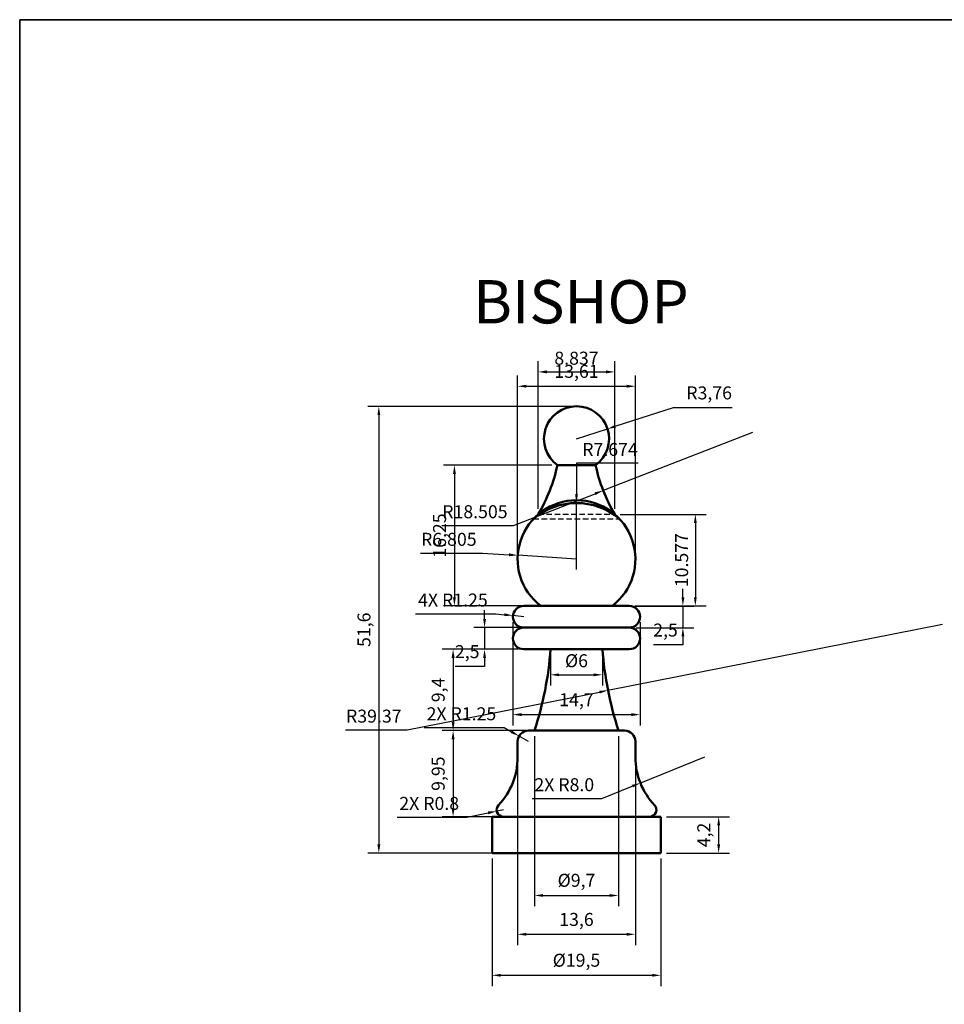
# Model space of a CAD drawing. Units: millimetres. Extents: x 172 to 469, y -14 to 196.
# Tile 2 of 5: x 172 to 279, y 82 to 196. Entities that reach past the tile are written whole.
import ezdxf

# ---------------------------------------------------------------- set-up
doc = ezdxf.new("R2010")
doc.units = ezdxf.units.MM
doc.header["$LTSCALE"] = 0.1
doc.linetypes.add('HIDDEN', pattern=[9.525, 6.35, -3.175])
for name, color, linetype, lineweight in [('M-DIMS', 2, 'Continuous', 25), ('M-HIDN', 1, 'HIDDEN', 25), ('M-OUTL', 7, 'Continuous', 50), ('M-TEXT', 3, 'Continuous', 25), ('M-TTLB', 7, 'Continuous', 35)]:
    doc.layers.add(name, color=color, linetype=linetype, lineweight=lineweight)
doc.styles.get("Standard").update_dxf_attribs({"font": 'arial.ttf'})
doc.dimstyles.new('ISO-25', dxfattribs={"dimtxt": 1.5, "dimasz": 1, "dimexe": 1.25, "dimexo": 0.625, "dimtad": 1, "dimtoh": 1, "dimtxsty": 'Standard', "dimcen": 2.5, "dimadec": 0, "dimazin": 0, "dimtfac": 1, "dimtmove": 0, "dimatfit": 3, "dimfxl": 1, "dimarcsym": 0})

# ---------------------------------------------------------------- blocks, each defined once
blk = doc.blocks.new('*D1')
at = {"layer": 'Defpoints', "color": 0, "ltscale": 0.1, "transparency": 16777216}
for p in [(229.35, 126.91), (244.05, 126.91), (244.05, 115.61)]:
    blk.add_point(p, dxfattribs=at)
at = {"layer": 'M-DIMS', "color": 0, "lineweight": -2, "ltscale": 0.1, "transparency": 16777216}
for p, q in [((229.35, 126.29), (229.35, 114.36)), ((244.05, 126.29), (244.05, 114.36)), ((230.35, 115.61), (243.05, 115.61))]:
    blk.add_line(p, q, dxfattribs=at)
at = {"layer": 'M-DIMS', "color": 0, "ltscale": 0.1, "transparency": 16777216}
for points in [[(230.35, 115.78), (230.35, 115.44), (229.35, 115.61)], [(243.05, 115.78), (243.05, 115.44), (244.05, 115.61)]]:
    blk.add_solid(points, dxfattribs=at)
at = {"layer": 'M-DIMS', "color": 0, "ltscale": 0.1, "transparency": 16777216, "insert": (236.7, 117.14), "char_height": 1.5, "attachment_point": 5}
blk.add_mtext('14,7', dxfattribs=at)
blk = doc.blocks.new('*D2')
at = {"layer": 'Defpoints', "color": 0, "ltscale": 0.1, "transparency": 16777216}
for p in [(233.7, 123.16), (239.7, 123.16), (239.7, 120.21)]:
    blk.add_point(p, dxfattribs=at)
at = {"layer": 'M-DIMS', "color": 0, "lineweight": -2, "ltscale": 0.1, "transparency": 16777216}
for p, q in [((233.7, 122.54), (233.7, 118.96)), ((239.7, 122.54), (239.7, 118.96)), ((234.7, 120.21), (238.7, 120.21))]:
    blk.add_line(p, q, dxfattribs=at)
at = {"layer": 'M-DIMS', "color": 0, "ltscale": 0.1, "transparency": 16777216}
for points in [[(234.7, 120.37), (234.7, 120.04), (233.7, 120.21)], [(238.7, 120.37), (238.7, 120.04), (239.7, 120.21)]]:
    blk.add_solid(points, dxfattribs=at)
at = {"layer": 'M-DIMS', "color": 0, "ltscale": 0.1, "transparency": 16777216, "insert": (236.7, 121.64), "char_height": 1.5, "attachment_point": 5}
blk.add_mtext('%%C6', dxfattribs=at)
blk = doc.blocks.new('*D3')
at = {"layer": 'Defpoints', "color": 0, "ltscale": 0.1, "transparency": 16777216}
for p in [(243.51, 153.53), (229.9, 133.57), (243.51, 133.57)]:
    blk.add_point(p, dxfattribs=at)
at = {"layer": 'M-DIMS', "color": 0, "lineweight": -2, "ltscale": 0.1, "transparency": 16777216}
for p, q in [((229.9, 134.19), (229.9, 154.78)), ((243.51, 134.19), (243.51, 154.78)), ((230.9, 153.53), (242.51, 153.53))]:
    blk.add_line(p, q, dxfattribs=at)
at = {"layer": 'M-DIMS', "color": 0, "ltscale": 0.1, "transparency": 16777216}
for points in [[(230.9, 153.7), (230.9, 153.37), (229.9, 153.53)], [(242.51, 153.7), (242.51, 153.37), (243.51, 153.53)]]:
    blk.add_solid(points, dxfattribs=at)
at = {"layer": 'M-DIMS', "color": 0, "ltscale": 0.1, "transparency": 16777216, "insert": (236.7, 155.06), "char_height": 1.5, "attachment_point": 5}
blk.add_mtext('13,61', dxfattribs=at)
blk = doc.blocks.new('*D4')
at = {"layer": 'Defpoints', "color": 0, "ltscale": 0.1, "transparency": 16777216}
for p in [(226.95, 99.61), (246.45, 99.61), (246.45, 85.5)]:
    blk.add_point(p, dxfattribs=at)
at = {"layer": 'M-DIMS', "color": 0, "lineweight": -2, "ltscale": 0.1, "transparency": 16777216}
for p, q in [((226.95, 98.99), (226.95, 84.25)), ((246.45, 98.99), (246.45, 84.25)), ((227.95, 85.5), (245.45, 85.5))]:
    blk.add_line(p, q, dxfattribs=at)
at = {"layer": 'M-DIMS', "color": 0, "ltscale": 0.1, "transparency": 16777216}
for points in [[(227.95, 85.67), (227.95, 85.34), (226.95, 85.5)], [(245.45, 85.67), (245.45, 85.34), (246.45, 85.5)]]:
    blk.add_solid(points, dxfattribs=at)
at = {"layer": 'M-DIMS', "color": 0, "ltscale": 0.1, "transparency": 16777216, "insert": (236.7, 87.05), "char_height": 1.5, "attachment_point": 5}
blk.add_mtext('%%C19,5', dxfattribs=at)
blk = doc.blocks.new('*D5')
at = {"layer": 'Defpoints', "color": 0, "ltscale": 0.1, "transparency": 16777216}
for p in [(229.9, 111.6), (243.5, 111.6), (243.5, 90.24)]:
    blk.add_point(p, dxfattribs=at)
at = {"layer": 'M-DIMS', "color": 0, "lineweight": -2, "ltscale": 0.1, "transparency": 16777216}
for p, q in [((229.9, 110.97), (229.9, 88.99)), ((243.5, 110.97), (243.5, 88.99)), ((230.9, 90.24), (242.5, 90.24))]:
    blk.add_line(p, q, dxfattribs=at)
at = {"layer": 'M-DIMS', "color": 0, "ltscale": 0.1, "transparency": 16777216}
for points in [[(230.9, 90.4), (230.9, 90.07), (229.9, 90.24)], [(242.5, 90.4), (242.5, 90.07), (243.5, 90.24)]]:
    blk.add_solid(points, dxfattribs=at)
at = {"layer": 'M-DIMS', "color": 0, "ltscale": 0.1, "transparency": 16777216, "insert": (236.7, 91.76), "char_height": 1.5, "attachment_point": 5}
blk.add_mtext('13,6', dxfattribs=at)
blk = doc.blocks.new('*D6')
at = {"layer": 'Defpoints', "color": 0, "ltscale": 0.1, "transparency": 16777216}
for p in [(231.85, 113.76), (241.55, 113.76), (241.55, 94.72)]:
    blk.add_point(p, dxfattribs=at)
at = {"layer": 'M-DIMS', "color": 0, "lineweight": -2, "ltscale": 0.1, "transparency": 16777216}
for p, q in [((231.85, 113.14), (231.85, 93.47)), ((241.55, 113.14), (241.55, 93.47)), ((232.85, 94.72), (240.55, 94.72))]:
    blk.add_line(p, q, dxfattribs=at)
at = {"layer": 'M-DIMS', "color": 0, "ltscale": 0.1, "transparency": 16777216}
for points in [[(232.85, 94.89), (232.85, 94.56), (231.85, 94.72)], [(240.55, 94.89), (240.55, 94.56), (241.55, 94.72)]]:
    blk.add_solid(points, dxfattribs=at)
at = {"layer": 'M-DIMS', "color": 0, "ltscale": 0.1, "transparency": 16777216, "insert": (236.7, 96.28), "char_height": 1.5, "attachment_point": 5}
blk.add_mtext('%%C9,7', dxfattribs=at)
blk = doc.blocks.new('*D7')
at = {"layer": 'Defpoints', "color": 0, "ltscale": 0.1, "transparency": 16777216}
for p in [(242.97, 128.15), (242.97, 125.65), (248.99, 125.65)]:
    blk.add_point(p, dxfattribs=at)
at = {"layer": 'M-DIMS', "color": 0, "lineweight": -2, "ltscale": 0.1, "transparency": 16777216}
for p, q in [((248.99, 129.15), (248.99, 130.15)), ((243.59, 128.15), (250.24, 128.15)), ((248.99, 128.15), (248.99, 125.65)), ((243.59, 125.65), (250.24, 125.65)), ((248.99, 124.65), (248.99, 123.65)), ((248.99, 123.65), (245.6, 123.65))]:
    blk.add_line(p, q, dxfattribs=at)
at = {"layer": 'M-DIMS', "color": 0, "ltscale": 0.1, "transparency": 16777216}
for points in [[(248.83, 129.15), (249.16, 129.15), (248.99, 128.15)], [(248.83, 124.65), (249.16, 124.65), (248.99, 125.65)]]:
    blk.add_solid(points, dxfattribs=at)
at = {"layer": 'M-DIMS', "color": 0, "ltscale": 0.1, "transparency": 16777216, "insert": (246.98, 125.18), "char_height": 1.5, "attachment_point": 5}
blk.add_mtext('2,5', dxfattribs=at)
blk = doc.blocks.new('*D8')
at = {"layer": 'Defpoints', "color": 0, "ltscale": 0.1, "transparency": 16777216}
for p in [(233.31, 113.76), (222.45, 103.81), (233.31, 103.81)]:
    blk.add_point(p, dxfattribs=at)
at = {"layer": 'M-DIMS', "color": 0, "lineweight": -2, "ltscale": 0.1, "transparency": 16777216}
for p, q in [((232.69, 113.76), (221.2, 113.76)), ((222.45, 112.76), (222.45, 104.81)), ((232.69, 103.81), (221.2, 103.81))]:
    blk.add_line(p, q, dxfattribs=at)
at = {"layer": 'M-DIMS', "color": 0, "ltscale": 0.1, "transparency": 16777216}
for points in [[(222.28, 112.76), (222.62, 112.76), (222.45, 113.76)], [(222.28, 104.81), (222.62, 104.81), (222.45, 103.81)]]:
    blk.add_solid(points, dxfattribs=at)
at = {"layer": 'M-DIMS', "color": 0, "ltscale": 0.1, "transparency": 16777216, "insert": (220.92, 108.79), "char_height": 1.5, "attachment_point": 5, "rotation": 90}
blk.add_mtext('9,95', dxfattribs=at)
blk = doc.blocks.new('*D9')
at = {"layer": 'Defpoints', "color": 0, "ltscale": 0.1, "transparency": 16777216}
for p in [(230.6, 125.66), (226.08, 123.16), (230.6, 123.16)]:
    blk.add_point(p, dxfattribs=at)
at = {"layer": 'M-DIMS', "color": 0, "lineweight": -2, "ltscale": 0.1, "transparency": 16777216}
for p, q in [((226.08, 126.66), (226.08, 127.66)), ((229.98, 125.66), (224.83, 125.66)), ((226.08, 125.66), (226.08, 123.16)), ((229.98, 123.16), (224.83, 123.16)), ((226.08, 122.16), (226.08, 121.16)), ((226.08, 121.16), (222.69, 121.16))]:
    blk.add_line(p, q, dxfattribs=at)
at = {"layer": 'M-DIMS', "color": 0, "ltscale": 0.1, "transparency": 16777216}
for points in [[(225.92, 126.66), (226.25, 126.66), (226.08, 125.66)], [(225.92, 122.16), (226.25, 122.16), (226.08, 123.16)]]:
    blk.add_solid(points, dxfattribs=at)
at = {"layer": 'M-DIMS', "color": 0, "ltscale": 0.1, "transparency": 16777216, "insert": (224.08, 122.69), "char_height": 1.5, "attachment_point": 5}
blk.add_mtext('2,5', dxfattribs=at)
blk = doc.blocks.new('*D10')
at = {"layer": 'Defpoints', "color": 0, "ltscale": 0.1, "transparency": 16777216}
for p in [(230.6, 123.16), (222.45, 113.76), (231.09, 113.76)]:
    blk.add_point(p, dxfattribs=at)
at = {"layer": 'M-DIMS', "color": 0, "lineweight": -2, "ltscale": 0.1, "transparency": 16777216}
for p, q in [((229.98, 123.16), (221.2, 123.16)), ((222.45, 122.16), (222.45, 114.76)), ((230.46, 113.76), (221.2, 113.76))]:
    blk.add_line(p, q, dxfattribs=at)
at = {"layer": 'M-DIMS', "color": 0, "ltscale": 0.1, "transparency": 16777216}
for points in [[(222.28, 122.16), (222.62, 122.16), (222.45, 123.16)], [(222.28, 114.76), (222.62, 114.76), (222.45, 113.76)]]:
    blk.add_solid(points, dxfattribs=at)
at = {"layer": 'M-DIMS', "color": 0, "ltscale": 0.1, "transparency": 16777216, "insert": (220.92, 118.46), "char_height": 1.5, "attachment_point": 5, "rotation": 90}
blk.add_mtext('9,4', dxfattribs=at)
blk = doc.blocks.new('*D11')
at = {"layer": 'Defpoints', "color": 0, "ltscale": 0.1, "transparency": 16777216}
for p in [(234.49, 144.41), (222.6, 128.16), (234.49, 128.16)]:
    blk.add_point(p, dxfattribs=at)
at = {"layer": 'M-DIMS', "color": 0, "lineweight": -2, "ltscale": 0.1, "transparency": 16777216}
for p, q in [((233.87, 144.41), (221.35, 144.41)), ((222.6, 143.41), (222.6, 129.16)), ((233.87, 128.16), (221.35, 128.16))]:
    blk.add_line(p, q, dxfattribs=at)
at = {"layer": 'M-DIMS', "color": 0, "ltscale": 0.1, "transparency": 16777216}
for points in [[(222.44, 143.41), (222.77, 143.41), (222.6, 144.41)], [(222.44, 129.16), (222.77, 129.16), (222.6, 128.16)]]:
    blk.add_solid(points, dxfattribs=at)
at = {"layer": 'M-DIMS', "color": 0, "ltscale": 0.1, "transparency": 16777216, "insert": (221.08, 136.29), "char_height": 1.5, "attachment_point": 5, "rotation": 90}
blk.add_mtext('16,25', dxfattribs=at)
blk = doc.blocks.new('*D12')
at = {"layer": 'Defpoints', "color": 0, "ltscale": 0.1, "transparency": 16777216}
for p in [(236.7, 151.21), (213.87, 99.61), (236.7, 99.61)]:
    blk.add_point(p, dxfattribs=at)
at = {"layer": 'M-DIMS', "color": 0, "lineweight": -2, "ltscale": 0.1, "transparency": 16777216}
for p, q in [((236.08, 151.21), (212.62, 151.21)), ((213.87, 150.21), (213.87, 100.61)), ((236.08, 99.61), (212.62, 99.61))]:
    blk.add_line(p, q, dxfattribs=at)
at = {"layer": 'M-DIMS', "color": 0, "ltscale": 0.1, "transparency": 16777216}
for points in [[(213.71, 150.21), (214.04, 150.21), (213.87, 151.21)], [(213.71, 100.61), (214.04, 100.61), (213.87, 99.61)]]:
    blk.add_solid(points, dxfattribs=at)
at = {"layer": 'M-DIMS', "color": 0, "ltscale": 0.1, "transparency": 16777216, "insert": (212.35, 125.41), "char_height": 1.5, "attachment_point": 5, "rotation": 90}
blk.add_mtext('51,6', dxfattribs=at)
blk = doc.blocks.new('*D13')
at = {"layer": 'Defpoints', "color": 0, "ltscale": 0.1, "transparency": 16777216}
for p in [(240.28, 148.61), (236.7, 147.45)]:
    blk.add_point(p, dxfattribs=at)
at = {"layer": 'M-DIMS', "color": 0, "lineweight": -2, "ltscale": 0.1, "transparency": 16777216}
for p, q in [((247.85, 151.05), (241.23, 148.91)), ((254.69, 151.05), (247.85, 151.05)), ((236.7, 147.45), (240.28, 148.61))]:
    blk.add_line(p, q, dxfattribs=at)
at = {"layer": 'M-DIMS', "color": 0, "ltscale": 0.1, "transparency": 16777216}
blk.add_solid([(241.18, 149.07), (241.28, 148.76), (240.28, 148.61)], dxfattribs=at)
at = {"layer": 'M-DIMS', "color": 0, "ltscale": 0.1, "transparency": 16777216, "insert": (252.02, 152.57), "char_height": 1.5, "attachment_point": 5}
blk.add_mtext('R3,76', dxfattribs=at)
blk = doc.blocks.new('*D14')
at = {"layer": 'Defpoints', "color": 0, "ltscale": 0.1, "transparency": 16777216}
for p in [(246.45, 103.81), (246.45, 99.61), (253.12, 99.61)]:
    blk.add_point(p, dxfattribs=at)
at = {"layer": 'M-DIMS', "color": 0, "lineweight": -2, "ltscale": 0.1, "transparency": 16777216}
for p, q in [((247.08, 103.81), (254.37, 103.81)), ((253.12, 102.81), (253.12, 100.61)), ((247.08, 99.61), (254.37, 99.61))]:
    blk.add_line(p, q, dxfattribs=at)
at = {"layer": 'M-DIMS', "color": 0, "ltscale": 0.1, "transparency": 16777216}
for points in [[(252.96, 102.81), (253.29, 102.81), (253.12, 103.81)], [(252.96, 100.61), (253.29, 100.61), (253.12, 99.61)]]:
    blk.add_solid(points, dxfattribs=at)
at = {"layer": 'M-DIMS', "color": 0, "ltscale": 0.1, "transparency": 16777216, "insert": (251.6, 101.71), "char_height": 1.5, "attachment_point": 5, "rotation": 90}
blk.add_mtext('4,2', dxfattribs=at)
blk = doc.blocks.new('*D59')
at = {"layer": 'Defpoints', "color": 0, "ltscale": 0.1, "transparency": 16777216}
for p in [(241.12, 138.74), (242.8, 128.16), (250.43, 128.16)]:
    blk.add_point(p, dxfattribs=at)
at = {"layer": 'M-DIMS', "color": 0, "lineweight": -2, "ltscale": 0.1, "transparency": 16777216}
for p, q in [((241.75, 138.74), (251.68, 138.74)), ((250.43, 137.74), (250.43, 129.16)), ((243.43, 128.16), (251.68, 128.16))]:
    blk.add_line(p, q, dxfattribs=at)
at = {"layer": 'M-DIMS', "color": 0, "ltscale": 0.1, "transparency": 16777216}
for points in [[(250.26, 137.74), (250.59, 137.74), (250.43, 138.74)], [(250.26, 129.16), (250.59, 129.16), (250.43, 128.16)]]:
    blk.add_solid(points, dxfattribs=at)
at = {"layer": 'M-DIMS', "color": 0, "ltscale": 0.1, "transparency": 16777216, "insert": (249.04, 133.45), "char_height": 1.5, "attachment_point": 5, "rotation": 90}
blk.add_mtext('10.577', dxfattribs=at)
blk = doc.blocks.new('*D60')
at = {"layer": 'Defpoints', "color": 0, "ltscale": 0.1, "transparency": 16777216}
for p in [(241.12, 155.19), (232.28, 138.74), (241.12, 138.74)]:
    blk.add_point(p, dxfattribs=at)
at = {"layer": 'M-DIMS', "color": 0, "lineweight": -2, "ltscale": 0.1, "transparency": 16777216}
for p, q in [((232.28, 139.37), (232.28, 156.44)), ((241.12, 139.37), (241.12, 156.44)), ((233.28, 155.19), (240.12, 155.19))]:
    blk.add_line(p, q, dxfattribs=at)
at = {"layer": 'M-DIMS', "color": 0, "ltscale": 0.1, "transparency": 16777216}
for points in [[(233.28, 155.36), (233.28, 155.02), (232.28, 155.19)], [(240.12, 155.36), (240.12, 155.02), (241.12, 155.19)]]:
    blk.add_solid(points, dxfattribs=at)
at = {"layer": 'M-DIMS', "color": 0, "ltscale": 0.1, "transparency": 16777216, "insert": (236.7, 156.58), "char_height": 1.5, "attachment_point": 5}
blk.add_mtext('8.837', dxfattribs=at)
blk = doc.blocks.new('*D66')
at = {"layer": 'Defpoints', "color": 0, "ltscale": 0.1, "transparency": 16777216}
for p in [(278.97, 126.01), (240.34, 118.41)]:
    blk.add_point(p, dxfattribs=at)
at = {"layer": 'M-DIMS', "color": 0, "lineweight": -2, "ltscale": 0.1, "transparency": 16777216}
for p, q in [((278.97, 126.01), (240.34, 118.41)), ((217.16, 113.85), (239.36, 118.21)), ((210.04, 113.85), (217.16, 113.85))]:
    blk.add_line(p, q, dxfattribs=at)
at = {"layer": 'M-DIMS', "color": 0, "ltscale": 0.1, "transparency": 16777216}
blk.add_solid([(239.33, 118.38), (239.39, 118.05), (240.34, 118.41)], dxfattribs=at)
at = {"layer": 'M-DIMS', "color": 0, "ltscale": 0.1, "transparency": 16777216, "insert": (213.29, 115.24), "char_height": 1.5, "attachment_point": 5}
blk.add_mtext('R39.37', dxfattribs=at)
blk = doc.blocks.new('*D67')
at = {"layer": 'Defpoints', "color": 0, "ltscale": 0.1, "transparency": 16777216}
for p in [(257.03, 148.19), (239.78, 141.49)]:
    blk.add_point(p, dxfattribs=at)
at = {"layer": 'M-DIMS', "color": 0, "lineweight": -2, "ltscale": 0.1, "transparency": 16777216}
for p, q in [((257.03, 148.19), (239.78, 141.49)), ((229.44, 137.46), (238.85, 141.12)), ((221.14, 137.46), (229.44, 137.46))]:
    blk.add_line(p, q, dxfattribs=at)
at = {"layer": 'M-DIMS', "color": 0, "ltscale": 0.1, "transparency": 16777216}
blk.add_solid([(238.79, 141.28), (238.91, 140.97), (239.78, 141.49)], dxfattribs=at)
at = {"layer": 'M-DIMS', "color": 0, "ltscale": 0.1, "transparency": 16777216, "insert": (224.97, 138.85), "char_height": 1.5, "attachment_point": 5}
blk.add_mtext('R18.505', dxfattribs=at)
blk = doc.blocks.new('*D68')
at = {"layer": 'Defpoints', "color": 0, "ltscale": 0.1, "transparency": 16777216}
for p in [(251.5, 110.69), (244.08, 107.71)]:
    blk.add_point(p, dxfattribs=at)
at = {"layer": 'M-DIMS', "color": 0, "lineweight": -2, "ltscale": 0.1, "transparency": 16777216}
for p, q in [((251.5, 110.69), (244.08, 107.71)), ((239.62, 105.93), (243.15, 107.34)), ((231.58, 105.93), (239.62, 105.93))]:
    blk.add_line(p, q, dxfattribs=at)
at = {"layer": 'M-DIMS', "color": 0, "ltscale": 0.1, "transparency": 16777216}
blk.add_solid([(243.09, 107.5), (243.21, 107.19), (244.08, 107.71)], dxfattribs=at)
at = {"layer": 'M-DIMS', "color": 0, "ltscale": 0.1, "transparency": 16777216, "insert": (235.29, 107.32), "char_height": 1.5, "attachment_point": 5}
blk.add_mtext('2X R8.0', dxfattribs=at)
blk = doc.blocks.new('*D69')
at = {"layer": 'Defpoints', "color": 0, "ltscale": 0.1, "transparency": 16777216}
for p in [(236.7, 140.04), (236.7, 132.37)]:
    blk.add_point(p, dxfattribs=at)
at = {"layer": 'M-DIMS', "color": 0, "lineweight": -2, "ltscale": 0.1, "transparency": 16777216}
for p, q in [((243.82, 144.64), (236.7, 144.64)), ((236.7, 144.64), (236.7, 141.04)), ((236.7, 132.37), (236.7, 140.04))]:
    blk.add_line(p, q, dxfattribs=at)
at = {"layer": 'M-DIMS', "color": 0, "ltscale": 0.1, "transparency": 16777216}
blk.add_solid([(236.54, 141.04), (236.87, 141.04), (236.7, 140.04)], dxfattribs=at)
at = {"layer": 'M-DIMS', "color": 0, "ltscale": 0.1, "transparency": 16777216, "insert": (240.57, 146.04), "char_height": 1.5, "attachment_point": 5}
blk.add_mtext('R7.674', dxfattribs=at)
blk = doc.blocks.new('*D70')
at = {"layer": 'Defpoints', "color": 0, "ltscale": 0.1, "transparency": 16777216}
for p in [(229.91, 134.01), (236.7, 133.57)]:
    blk.add_point(p, dxfattribs=at)
at = {"layer": 'M-DIMS', "color": 0, "lineweight": -2, "ltscale": 0.1, "transparency": 16777216}
for p, q in [((218.7, 134.27), (225.84, 134.27)), ((225.84, 134.27), (228.91, 134.07)), ((236.7, 133.57), (229.91, 134.01))]:
    blk.add_line(p, q, dxfattribs=at)
at = {"layer": 'M-DIMS', "color": 0, "ltscale": 0.1, "transparency": 16777216}
blk.add_solid([(228.92, 134.24), (228.9, 133.9), (229.91, 134.01)], dxfattribs=at)
at = {"layer": 'M-DIMS', "color": 0, "ltscale": 0.1, "transparency": 16777216, "insert": (221.96, 135.66), "char_height": 1.5, "attachment_point": 5}
blk.add_mtext('R6.805', dxfattribs=at)
blk = doc.blocks.new('*D71')
at = {"layer": 'Defpoints', "color": 0, "ltscale": 0.1, "transparency": 16777216}
for p in [(227.49, 104.46), (228.27, 104.61)]:
    blk.add_point(p, dxfattribs=at)
at = {"layer": 'M-DIMS', "color": 0, "lineweight": -2, "ltscale": 0.1, "transparency": 16777216}
for p, q in [((215.98, 103.77), (224.03, 103.77)), ((224.03, 103.77), (226.51, 104.26)), ((228.27, 104.61), (227.49, 104.46))]:
    blk.add_line(p, q, dxfattribs=at)
at = {"layer": 'M-DIMS', "color": 0, "ltscale": 0.1, "transparency": 16777216}
blk.add_solid([(226.48, 104.43), (226.54, 104.1), (227.49, 104.46)], dxfattribs=at)
at = {"layer": 'M-DIMS', "color": 0, "ltscale": 0.1, "transparency": 16777216, "insert": (219.69, 105.16), "char_height": 1.5, "attachment_point": 5}
blk.add_mtext('2X R0.8', dxfattribs=at)
blk = doc.blocks.new('*D72')
at = {"layer": 'Defpoints', "color": 0, "ltscale": 0.1, "transparency": 16777216}
for p in [(230.07, 113.13), (231.15, 112.51)]:
    blk.add_point(p, dxfattribs=at)
at = {"layer": 'M-DIMS', "color": 0, "lineweight": -2, "ltscale": 0.1, "transparency": 16777216}
for p, q in [((219.11, 114.12), (228.33, 114.12)), ((228.33, 114.12), (229.2, 113.63)), ((231.15, 112.51), (230.07, 113.13))]:
    blk.add_line(p, q, dxfattribs=at)
at = {"layer": 'M-DIMS', "color": 0, "ltscale": 0.1, "transparency": 16777216}
blk.add_solid([(229.28, 113.77), (229.11, 113.48), (230.07, 113.13)], dxfattribs=at)
at = {"layer": 'M-DIMS', "color": 0, "ltscale": 0.1, "transparency": 16777216, "insert": (223.41, 115.51), "char_height": 1.5, "attachment_point": 5}
blk.add_mtext('2X R1.25', dxfattribs=at)
blk = doc.blocks.new('*D73')
at = {"layer": 'Defpoints', "color": 0, "ltscale": 0.1, "transparency": 16777216}
for p in [(229.36, 127.05), (230.6, 126.91)]:
    blk.add_point(p, dxfattribs=at)
at = {"layer": 'M-DIMS', "color": 0, "lineweight": -2, "ltscale": 0.1, "transparency": 16777216}
for p, q in [((218.12, 127.26), (227.37, 127.26)), ((227.37, 127.26), (228.37, 127.15)), ((230.6, 126.91), (229.36, 127.05))]:
    blk.add_line(p, q, dxfattribs=at)
at = {"layer": 'M-DIMS', "color": 0, "ltscale": 0.1, "transparency": 16777216}
blk.add_solid([(228.38, 127.32), (228.35, 126.99), (229.36, 127.05)], dxfattribs=at)
at = {"layer": 'M-DIMS', "color": 0, "ltscale": 0.1, "transparency": 16777216, "insert": (222.43, 128.65), "char_height": 1.5, "attachment_point": 5}
blk.add_mtext('4X R1.25', dxfattribs=at)

msp = doc.modelspace()

# ---------------------------------------------------------------- linework, layer by layer
at = {"layer": 'M-HIDN'}
for p, q in [((232.2842, 138.7422), (241.1216, 138.7422)), ((231.7242, 138.206), (241.6815, 138.206))]:
    msp.add_line(p, q, dxfattribs=at)
at = {"layer": 'M-OUTL'}
for p, q in [((234.4902, 144.4148), (238.9156, 144.4148)), ((234.4902, 144.4148), (238.9156, 144.4148)), ((230.6029, 128.1648), (242.8029, 128.1648)), ((230.6029, 125.6648), (242.8029, 125.6648)), ((242.8029, 125.6648), (230.6029, 125.6648)), ((242.8029, 123.1648), (230.6029, 123.1648)), ((242.2529, 113.7648), (231.1529, 113.7648)), ((229.9029, 110.6851), (229.9029, 112.5148)), ((243.5029, 110.6851), (243.5029, 112.5148)), ((243.5029, 110.6851), (243.5029, 112.5148)), ((246.4529, 103.8148), (226.9529, 103.8148)), ((226.9529, 103.8148), (226.9529, 99.6148)), ((246.4529, 99.6148), (246.4529, 103.8148)), ((226.9529, 99.6148), (246.4529, 99.6148))]:
    msp.add_line(p, q, dxfattribs=at)
for centre, radius, start, end in [((236.7029, 147.4548), 3.76, 306.049329, 233.950671), ((216.375, 148.1943), 18.5052, 329.284134, 348.215178), ((257.0307, 148.1943), 18.5052, 191.784822, 210.715866), ((236.7029, 133.5669), 6.805, 307.453946, 232.546054), ((236.7029, 132.3667), 7.6736, 49.54898, 130.45102), ((230.6029, 126.9148), 1.25, 90, 270), ((242.8029, 126.9148), 1.25, 270, 90), ((230.6029, 124.4148), 1.25, 90, 270), ((242.8029, 124.4148), 1.25, 270, 90), ((194.4322, 126.0116), 39.3738, 341.878165, 355.853837), ((278.9736, 126.0116), 39.3738, 184.146163, 198.121835), ((231.1529, 112.5148), 1.25, 90, 180), ((242.2529, 112.5148), 1.25, 360, 90), ((221.9029, 110.6851), 8, 316.38585, 0), ((251.5029, 110.6851), 8, 180, 223.61415), ((228.2741, 104.6148), 0.8, 136.38585, 270), ((245.1317, 104.6148), 0.8, 270, 43.61415)]:
    msp.add_arc(centre, radius, start, end, dxfattribs=at)
at = {"layer": 'M-TTLB', "ltscale": 0.1}
msp.add_lwpolyline([(172.3921, 195.8665), (469.3921, 195.8665), (469.3921, -14.1335), (172.3921, -14.1335)], close=True, dxfattribs=at)

# ---------------------------------------------------------------- texts
at = {"layer": 'M-TEXT', "ltscale": 0.1, "insert": (215.1128, 165.7874), "char_height": 5, "attachment_point": 1}
msp.add_mtext_dynamic_manual_height_columns('\\pxqc;BISHOP', width=44.206943, gutter_width=12.5, heights=[0], dxfattribs=at)

# ---------------------------------------------------------------- dimensions: what is measured, and where the dimension line sits
at = {"layer": 'M-DIMS', "ltscale": 0.1}
for base, p1, p2, override, picture, middle in [((241.1216, 155.1898), (232.2842, 138.7422), (241.1216, 138.7422), {"dimdec": 3, "dimlfac": 1, "dimrnd": 0, "dimzin": 0, "dimdsep": 46, "dimlunit": 2}, '*D60', (236.7029, 156.5812)), ((243.5079, 153.5317), (229.8979, 133.5669), (243.5079, 133.5669), {"dimclrd": 0, "dimclre": 0, "dimclrt": 0}, '*D3', (236.7029, 155.0581)), ((244.0529, 115.6108), (229.3529, 126.9148), (244.0529, 126.9148), {"dimclrd": 0, "dimclre": 0, "dimclrt": 0}, '*D1', (236.7029, 117.1372))]:
    dim = msp.add_linear_dim(base=base, p1=p1, p2=p2, dimstyle='ISO-25', override=override, dxfattribs=at)
    dim.commit()
    dim.dimension.update_dxf_attribs({"geometry": picture, "text_midpoint": middle})
for center, mpoint, override, picture, middle in [((236.7029, 147.4548), (240.2817, 148.6081), {"dimclrd": 0, "dimclre": 0, "dimclrt": 0}, '*D13', (252.0242, 151.0454)), ((257.0307, 148.1943), (239.7839, 141.4869), {"dimdec": 3, "dimlfac": 1, "dimrnd": 0, "dimzin": 0, "dimdsep": 46, "dimlunit": 2}, '*D67', (224.9738, 137.4625)), ((236.7029, 132.3667), (236.703, 140.0403), {"dimdec": 3, "dimlfac": 1, "dimrnd": 0, "dimzin": 0, "dimdsep": 46, "dimlunit": 2}, '*D69', (240.5736, 144.6445)), ((236.7029, 133.5669), (229.912, 134.0057), {"dimdec": 3, "dimlfac": 1, "dimrnd": 0, "dimzin": 0, "dimdsep": 46, "dimlunit": 2}, '*D70', (225.8375, 134.2689)), ((278.9736, 126.0116), (240.341, 118.408), {"dimdec": 2, "dimlfac": 1, "dimrnd": 0, "dimzin": 0, "dimdsep": 46, "dimlunit": 2}, '*D66', (217.1614, 113.8458))]:
    dim = msp.add_radius_dim(center=center, mpoint=mpoint, dimstyle='ISO-25', override=override, dxfattribs=at)
    dim.commit()
    dim.dimension.update_dxf_attribs({"geometry": picture, "text_midpoint": middle, "dimtype": 164})
for base, p1, p2, override, picture, middle in [((213.8725, 99.6148), (236.7029, 151.2148), (236.7029, 99.6148), {"dimclrd": 0, "dimclre": 0, "dimclrt": 0}, '*D12', (212.346, 125.4148)), ((222.6032, 128.1648), (234.4902, 144.4148), (234.4902, 128.1648), {"dimclrd": 0, "dimclre": 0, "dimclrt": 0}, '*D11', (221.0768, 136.2898)), ((250.4279, 128.1648), (241.1216, 138.7422), (242.8029, 128.1648), {"dimdec": 3, "dimlfac": 1, "dimrnd": 0, "dimzin": 0, "dimdsep": 46, "dimlunit": 2}, '*D59', (249.037, 133.4535)), ((248.9921, 125.6541), (242.9664, 128.1541), (242.9664, 125.6541), {"dimclrd": 0, "dimclre": 0, "dimclrt": 0}, '*D7', (246.9832, 125.1805)), ((226.0841, 123.1648), (230.6029, 125.6648), (230.6029, 123.1648), {"dimclrd": 0, "dimclre": 0, "dimclrt": 0}, '*D9', (224.0753, 122.6913)), ((222.4508, 113.7632), (230.6029, 123.1648), (231.0884, 113.7632), {"dimclrd": 0, "dimclre": 0, "dimclrt": 0}, '*D10', (220.9243, 118.464)), ((222.4508, 103.8148), (233.3138, 113.7648), (233.3138, 103.8148), {"dimclrd": 0, "dimclre": 0, "dimclrt": 0}, '*D8', (220.9243, 108.7898)), ((253.1231, 99.6148), (246.4529, 103.8148), (246.4529, 99.6148), {"dimclrd": 0, "dimclre": 0, "dimclrt": 0}, '*D14', (251.5967, 101.7148))]:
    dim = msp.add_linear_dim(base=base, p1=p1, p2=p2, angle=90, dimstyle='ISO-25', override=override, dxfattribs=at)
    dim.commit()
    dim.dimension.update_dxf_attribs({"geometry": picture, "text_midpoint": middle})
for center, mpoint, text, override, picture, middle in [((230.6029, 126.9148), (229.3599, 127.0467), '4X <>', {"dimdec": 2, "dimlfac": 1, "dimrnd": 0, "dimzin": 0, "dimdsep": 46, "dimlunit": 2}, '*D73', (222.4327, 128.6485)), ((231.1529, 112.5148), (230.0664, 113.1329), '2X <>', {"dimdec": 2, "dimlfac": 1, "dimrnd": 0, "dimzin": 0, "dimdsep": 46, "dimlunit": 2}, '*D72', (223.4071, 115.5126)), ((228.2741, 104.6148), (227.4896, 104.4579), '2X <>', {"dimdec": 1, "dimlfac": 1, "dimrnd": 0, "dimzin": 0, "dimdsep": 46, "dimlunit": 2}, '*D71', (219.6924, 105.1561))]:
    dim = msp.add_radius_dim(center=center, mpoint=mpoint, text=text, dimstyle='ISO-25', override=override, dxfattribs=at)
    dim.commit()
    dim.dimension.update_dxf_attribs({"geometry": picture, "text_midpoint": middle})
dim = msp.add_linear_dim(base=(239.7029, 120.2077), p1=(233.7029, 123.1648), p2=(239.7029, 123.1648), text='%%C<>', dimstyle='ISO-25', override={"dimclrd": 0, "dimclre": 0, "dimclrt": 0}, dxfattribs=at)
dim.commit()
dim.dimension.update_dxf_attribs({"geometry": '*D2', "text_midpoint": (236.7029, 121.6405)})
for base, p1, p2, picture, middle in [((241.5529, 94.724), (231.8529, 113.7648), (241.5529, 113.7648), '*D6', (236.7029, 94.724)), ((246.4529, 85.5032), (226.9529, 99.6148), (246.4529, 99.6148), '*D4', (236.7029, 85.5032))]:
    dim = msp.add_linear_dim(base=base, p1=p1, p2=p2, text='%%C<>', dimstyle='ISO-25', override={"dimclrd": 0, "dimclre": 0, "dimclrt": 0}, dxfattribs=at)
    dim.commit()
    dim.dimension.update_dxf_attribs({"geometry": picture, "text_midpoint": middle, "dimtype": 160})
dim = msp.add_linear_dim(base=(243.5029, 90.2382), p1=(229.9029, 111.6), p2=(243.5029, 111.6), dimstyle='ISO-25', override={"dimclrd": 0, "dimclre": 0, "dimclrt": 0}, dxfattribs=at)
dim.commit()
dim.dimension.update_dxf_attribs({"geometry": '*D5', "text_midpoint": (236.7029, 90.2382), "dimtype": 160})
dim = msp.add_radius_dim(center=(251.5029, 110.6851), mpoint=(244.0754, 107.7132), text='2X <>', dimstyle='ISO-25', override={"dimdec": 1, "dimlfac": 1, "dimrnd": 0, "dimzin": 0, "dimdsep": 46, "dimlunit": 2}, dxfattribs=at)
dim.commit()
dim.dimension.update_dxf_attribs({"geometry": '*D68', "text_midpoint": (235.2889, 105.93), "dimtype": 164})

doc.saveas('drawing.dxf')
